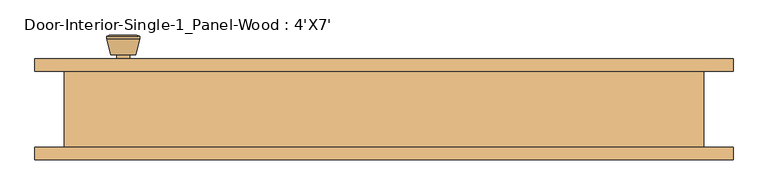
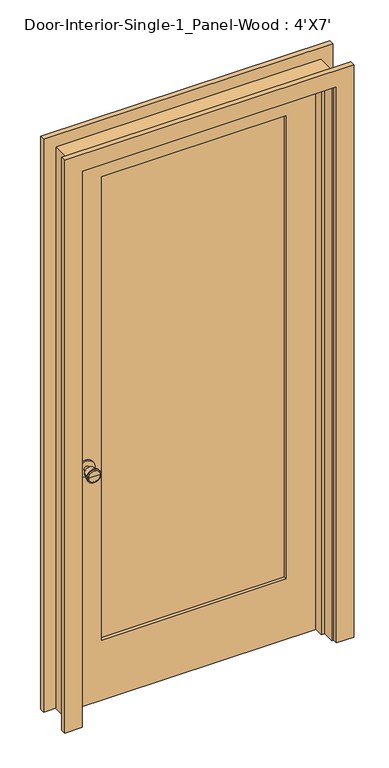
"""IFC4 building model written with IfcOpenShell, lengths in millimetres: door geometry, Door-Interior-Single-1_Panel-Wood : 4'X7'."""

from ifc_helpers import new_model, si_unit, point, frame, frame_2d, origin, place, context, project, spatial, polyline, circle_curve, trimmed, segment, composite_curve, outline, extrude, faceted_brep, source, transform, mapped, element, save
from ifc_brep_helpers import plane_surface, cylinder_surface, revolved_surface, advanced_brep


def door_interior_single_1_panel_wood_4_x7_3c6ab76a(model_context):
    return source(origin(), model_context, "Body", "SolidModel", [
        advanced_brep(
        [(-393.7, 13.05, 914.4), (-383.7, 13.05, 914.4), (-403.7, 13.05, 914.4), (-373.2241324, -35.95, 914.4), (-393.7, -35.95, 914.4), (-414.1758676, -35.95, 914.4), (-368.7, -34.1221319, 914.4), (-418.7, -34.1221319, 914.4), (-368.7, -30.6584537, 914.4), (-418.7, -30.6584537, 914.4), (-375.063764, -5.95, 914.4), (-412.336236, -5.95, 914.4), (-383.7, -5.95, 914.4), (-403.7, -5.95, 914.4)],
        [
            (0, 1),
            (1, 2, circle_curve(frame((-393.7, 13.05, 914.4), z_axis=(0.0, 1.0, 0.0), x_axis=(-1.0, 0.0, 0.0)), 10.0)),
            (2, 0),
            (2, 1, circle_curve(frame((-393.7, 13.05, 914.4), z_axis=(0.0, 1.0, 0.0), x_axis=(-1.0, 0.0, 0.0)), 10.0)),
            (3, 4),
            (4, 5),
            (5, 3, circle_curve(frame((-393.7, -35.95, 914.4), z_axis=(0.0, -1.0, 0.0), x_axis=(-1.0, 0.0, 0.0)), 20.4758676)),
            (3, 5, circle_curve(frame((-393.7, -35.95, 914.4), z_axis=(0.0, -1.0, 0.0), x_axis=(-1.0, 0.0, 0.0)), 20.4758676)),
            (6, 3),
            (5, 7),
            (7, 6, circle_curve(frame((-393.7, -34.1221319, 914.4), z_axis=(0.0, -1.0, 0.0), x_axis=(-1.0, 0.0, 0.0)), 25.0)),
            (6, 7, circle_curve(frame((-393.7, -34.1221319, 914.4), z_axis=(0.0, -1.0, 0.0), x_axis=(-1.0, 0.0, 0.0)), 25.0)),
            (8, 6),
            (7, 9),
            (9, 8, circle_curve(frame((-393.7, -30.6584537, 914.4), z_axis=(0.0, -1.0, 0.0), x_axis=(-1.0, 0.0, 0.0)), 25.0)),
            (8, 9, circle_curve(frame((-393.7, -30.6584537, 914.4), z_axis=(0.0, -1.0, 0.0), x_axis=(-1.0, 0.0, 0.0)), 25.0)),
            (10, 8),
            (9, 11),
            (11, 10, circle_curve(frame((-393.7, -5.95, 914.4), z_axis=(0.0, -1.0, 0.0), x_axis=(-1.0, 0.0, 0.0)), 18.636236)),
            (10, 11, circle_curve(frame((-393.7, -5.95, 914.4), z_axis=(0.0, -1.0, 0.0), x_axis=(-1.0, 0.0, 0.0)), 18.636236)),
            (12, 10),
            (11, 13),
            (13, 12, circle_curve(frame((-393.7, -5.95, 914.4), z_axis=(0.0, -1.0, 0.0), x_axis=(-1.0, 0.0, 0.0)), 10.0)),
            (12, 13, circle_curve(frame((-393.7, -5.95, 914.4), z_axis=(0.0, -1.0, 0.0), x_axis=(-1.0, 0.0, 0.0)), 10.0)),
            (1, 12),
            (13, 2),
        ],
        [
            plane_surface(frame((-393.7, 13.05, 914.4), z_axis=(0.0, 1.0, 0.0), x_axis=(-1.0, 0.0, 0.0))),
            plane_surface(frame((-393.7, -35.95, 914.4), z_axis=(0.0, -1.0, 0.0), x_axis=(-1.0, 0.0, 0.0))),
            revolved_surface(polyline([(-414.1758676, -35.95, 914.4), (-418.7, -34.1221319, 914.4)]), (-393.7, 13.05, 914.4), (0.0, 1.0, 0.0)),
            cylinder_surface(frame((-393.7, 13.05, 914.4), z_axis=(0.0, 1.0, 0.0), x_axis=(-1.0, 0.0, 0.0)), 25.0),
            revolved_surface(polyline([(-418.7, -30.6584537, 914.4), (-412.336236, -5.95, 914.4)]), (-393.7, 13.05, 914.4), (0.0, 1.0, 0.0)),
            plane_surface(frame((-393.7, -5.95, 914.4), z_axis=(0.0, 1.0, 0.0), x_axis=(-1.0, 0.0, 0.0))),
            cylinder_surface(frame((-393.7, 13.05, 914.4), z_axis=(0.0, 1.0, 0.0), x_axis=(-1.0, 0.0, 0.0)), 10.0),
        ],
        [
            (0, [[1, 2, 3]]),
            (0, [[-3, 4, -1]]),
            (1, [[5, 6, 7]]),
            (1, [[-6, -5, 8]]),
            (2, [[9, -7, 10, 11]]),
            (2, [[-10, -8, -9, 12]]),
            (3, [[13, -11, 14, 15]]),
            (3, [[-14, -12, -13, 16]]),
            (4, [[17, -15, 18, 19]]),
            (4, [[-18, -16, -17, 20]]),
            (5, [[21, -19, 22, 23]]),
            (5, [[-22, -20, -21, 24]]),
            (6, [[25, -23, 26, -2]]),
            (6, [[-26, -24, -25, -4]]),
        ],
    ),
        extrude(outline(composite_curve([segment(trimmed(circle_curve(frame_2d((914.4, -393.7)), 30.0), [point((914.4, -423.7))], [point((914.4, -363.7))], False, "CARTESIAN"), True, "CONTINUOUS"), segment(trimmed(circle_curve(frame_2d((914.4, -393.7)), 30.0), [point((914.4, -363.7))], [point((914.4, -423.7))], False, "CARTESIAN"), True, "CONTINUOUS")], self_intersect=False)), frame((0.0, 13.05, 0.0), z_axis=(0.0, 1.0, 0.0), x_axis=(0.0, 0.0, 1.0)), (0.0, 0.0, 1.0), 6.0),
        advanced_brep(
        [(-393.7, 59.975, 914.4), (-403.7, 59.975, 914.4), (-383.7, 59.975, 914.4), (-373.2241324, 108.975, 914.4), (-414.1758676, 108.975, 914.4), (-393.7, 108.975, 914.4), (-368.7, 107.1471319, 914.4), (-418.7, 107.1471319, 914.4), (-368.7, 103.6834537, 914.4), (-418.7, 103.6834537, 914.4), (-375.063764, 78.975, 914.4), (-412.336236, 78.975, 914.4), (-383.7, 78.975, 914.4), (-403.7, 78.975, 914.4)],
        [
            (0, 1),
            (1, 2, circle_curve(frame((-393.7, 59.975, 914.4), z_axis=(0.0, -1.0, 0.0), x_axis=(-1.0, 0.0, 0.0)), 10.0)),
            (2, 0),
            (2, 1, circle_curve(frame((-393.7, 59.975, 914.4), z_axis=(0.0, -1.0, 0.0), x_axis=(-1.0, 0.0, 0.0)), 10.0)),
            (3, 4, circle_curve(frame((-393.7, 108.975, 914.4), z_axis=(0.0, 1.0, 0.0), x_axis=(-1.0, 0.0, 0.0)), 20.4758676)),
            (4, 5),
            (5, 3),
            (4, 3, circle_curve(frame((-393.7, 108.975, 914.4), z_axis=(0.0, 1.0, 0.0), x_axis=(-1.0, 0.0, 0.0)), 20.4758676)),
            (6, 7, circle_curve(frame((-393.7, 107.1471319, 914.4), z_axis=(0.0, 1.0, 0.0), x_axis=(-1.0, 0.0, 0.0)), 25.0)),
            (7, 4),
            (3, 6),
            (7, 6, circle_curve(frame((-393.7, 107.1471319, 914.4), z_axis=(0.0, 1.0, 0.0), x_axis=(-1.0, 0.0, 0.0)), 25.0)),
            (8, 9, circle_curve(frame((-393.7, 103.6834537, 914.4), z_axis=(0.0, 1.0, 0.0), x_axis=(-1.0, 0.0, 0.0)), 25.0)),
            (9, 7),
            (6, 8),
            (9, 8, circle_curve(frame((-393.7, 103.6834537, 914.4), z_axis=(0.0, 1.0, 0.0), x_axis=(-1.0, 0.0, 0.0)), 25.0)),
            (10, 11, circle_curve(frame((-393.7, 78.975, 914.4), z_axis=(0.0, 1.0, 0.0), x_axis=(-1.0, 0.0, 0.0)), 18.636236)),
            (11, 9),
            (8, 10),
            (11, 10, circle_curve(frame((-393.7, 78.975, 914.4), z_axis=(0.0, 1.0, 0.0), x_axis=(-1.0, 0.0, 0.0)), 18.636236)),
            (12, 13, circle_curve(frame((-393.7, 78.975, 914.4), z_axis=(0.0, 1.0, 0.0), x_axis=(-1.0, 0.0, 0.0)), 10.0)),
            (13, 11),
            (10, 12),
            (13, 12, circle_curve(frame((-393.7, 78.975, 914.4), z_axis=(0.0, 1.0, 0.0), x_axis=(-1.0, 0.0, 0.0)), 10.0)),
            (1, 13),
            (12, 2),
        ],
        [
            plane_surface(frame((-393.7, 59.975, 914.4), z_axis=(0.0, -1.0, 0.0), x_axis=(-1.0, 0.0, 0.0))),
            plane_surface(frame((-393.7, 108.975, 914.4), z_axis=(0.0, 1.0, 0.0), x_axis=(-1.0, 0.0, 0.0))),
            revolved_surface(polyline([(-414.1758676, 108.975, 914.4), (-418.7, 107.1471319, 914.4)]), (-393.7, 59.975, 914.4), (0.0, -1.0, 0.0)),
            cylinder_surface(frame((-393.7, 59.975, 914.4), z_axis=(0.0, -1.0, 0.0), x_axis=(-1.0, 0.0, 0.0)), 25.0),
            revolved_surface(polyline([(-418.7, 103.6834537, 914.4), (-412.336236, 78.975, 914.4)]), (-393.7, 59.975, 914.4), (0.0, -1.0, 0.0)),
            plane_surface(frame((-393.7, 78.975, 914.4), z_axis=(0.0, -1.0, 0.0), x_axis=(-1.0, 0.0, 0.0))),
            cylinder_surface(frame((-393.7, 59.975, 914.4), z_axis=(0.0, -1.0, 0.0), x_axis=(-1.0, 0.0, 0.0)), 10.0),
        ],
        [
            (0, [[1, 2, 3]]),
            (0, [[-3, 4, -1]]),
            (1, [[5, 6, 7]]),
            (1, [[8, -7, -6]]),
            (2, [[9, 10, -5, 11]]),
            (2, [[12, -11, -8, -10]]),
            (3, [[13, 14, -9, 15]]),
            (3, [[16, -15, -12, -14]]),
            (4, [[17, 18, -13, 19]]),
            (4, [[20, -19, -16, -18]]),
            (5, [[21, 22, -17, 23]]),
            (5, [[24, -23, -20, -22]]),
            (6, [[-2, 25, -21, 26]]),
            (6, [[-4, -26, -24, -25]]),
        ],
    ),
        extrude(outline(composite_curve([segment(trimmed(circle_curve(frame_2d((914.4, -393.7)), 30.0), [point((914.4, -423.7))], [point((914.4, -363.7))], False, "CARTESIAN"), True, "CONTINUOUS"), segment(trimmed(circle_curve(frame_2d((914.4, -393.7)), 30.0), [point((914.4, -363.7))], [point((914.4, -423.7))], False, "CARTESIAN"), True, "CONTINUOUS")], self_intersect=False)), frame((0.0, 53.975, 0.0), z_axis=(0.0, 1.0, 0.0), x_axis=(0.0, 0.0, 1.0)), (0.0, 0.0, 1.0), 6.0),
        faceted_brep([(482.6, 53.975, 0.0), (482.6, -60.325, 0.0), (457.2, -60.325, 0.0), (457.2, -15.875, 0.0), (444.5, -15.875, 0.0), (444.5, 19.05, 0.0), (457.2, 19.05, 0.0), (457.2, 53.975, 0.0), (482.6, 53.975, 2159.0), (482.6, -60.325, 2159.0), (-482.6, -60.325, 2159.0), (-482.6, -60.325, 0.0), (-457.2, -60.325, 0.0), (-457.2, -60.325, 2133.6), (457.2, -60.325, 2133.6), (457.2, -15.875, 2133.6), (-457.2, -15.875, 2133.6), (-457.2, -15.875, 0.0), (-444.5, -15.875, 0.0), (-444.5, -15.875, 2120.9), (444.5, -15.875, 2120.9), (444.5, 19.05, 2120.9), (-444.5, 19.05, 2120.9), (-444.5, 19.05, 0.0), (-457.2, 19.05, 0.0), (-457.2, 19.05, 2133.6), (457.2, 19.05, 2133.6), (457.2, 53.975, 2133.6), (-457.2, 53.975, 2133.6), (-457.2, 53.975, 0.0), (-482.6, 53.975, 0.0), (-482.6, 53.975, 2159.0)], [[[0, 1, 2, 3, 4, 5, 6, 7]], [[1, 0, 8, 9]], [[2, 1, 9, 10, 11, 12, 13, 14]], [[3, 2, 14, 15]], [[4, 3, 15, 16, 17, 18, 19, 20]], [[5, 4, 20, 21]], [[6, 5, 21, 22, 23, 24, 25, 26]], [[7, 6, 26, 27]], [[0, 7, 27, 28, 29, 30, 31, 8]], [[9, 8, 31, 10]], [[15, 14, 13, 16]], [[21, 20, 19, 22]], [[27, 26, 25, 28]], [[30, 29, 24, 23, 18, 17, 12, 11]], [[10, 31, 30, 11]], [[16, 13, 12, 17]], [[22, 19, 18, 23]], [[28, 25, 24, 29]]]),
        extrude(outline(polyline([(2133.6, -457.2), (0.0, -457.2), (0.0, 457.2), (2133.6, 457.2), (2133.6, -457.2)]), holes=[polyline([(2014.5375, -336.55), (2014.5375, 336.55), (231.775, 336.55), (231.775, -336.55), (2014.5375, -336.55)])]), frame((0.0, 19.05, 0.0), z_axis=(0.0, 1.0, 0.0), x_axis=(0.0, 0.0, 1.0)), (0.0, 0.0, 1.0), 34.925),
        extrude(outline(polyline([(336.55, 30.6916667), (-336.55, 30.6916667), (-336.55, 42.3333333), (336.55, 42.3333333), (336.55, 30.6916667)])), frame((0.0, 0.0, 231.775), z_axis=(0.0, 0.0, 1.0), x_axis=(1.0, 0.0, 0.0)), (0.0, 0.0, 1.0), 1782.7625),
        extrude(outline(polyline([(0.0, 463.55), (0.0, 527.05), (2203.45, 527.05), (2203.45, -527.05), (0.0, -527.05), (0.0, -463.55), (2139.95, -463.55), (2139.95, 463.55), (0.0, 463.55)])), frame((0.0, 53.975, 0.0), z_axis=(0.0, 1.0, 0.0), x_axis=(0.0, 0.0, 1.0)), (0.0, 0.0, 1.0), 19.05),
        extrude(outline(polyline([(0.0, 463.55), (0.0, 527.05), (2203.45, 527.05), (2203.45, -527.05), (0.0, -527.05), (0.0, -463.55), (2139.95, -463.55), (2139.95, 463.55), (0.0, 463.55)])), frame((0.0, -79.375, 0.0), z_axis=(0.0, 1.0, 0.0), x_axis=(0.0, 0.0, 1.0)), (0.0, 0.0, 1.0), 19.05),
    ])


if __name__ == "__main__":
    model = new_model("IFC4")
    model_context = context("Model", 3, world=origin())
    ifc_project = project(units=[si_unit("LENGTHUNIT", "METRE", prefix="MILLI")], contexts=[model_context])
    site = spatial("IfcSite", under=ifc_project)
    building = spatial("IfcBuilding", under=site)
    placement = place(None, origin())
    door_interior_single_1_panel_wood_4_x7_shape = door_interior_single_1_panel_wood_4_x7_3c6ab76a(model_context)
    element("IfcDoor", 1, ObjectType="Door-Interior-Single-1_Panel-Wood : 4'X7'", at=placement, inside=building, context=model_context, shape_type="MappedRepresentation", body=[
        mapped(door_interior_single_1_panel_wood_4_x7_shape, transform((0.0, 0.0, 0.0), x_axis=(1.0, 0.0, 0.0), y_axis=(0.0, 1.0, 0.0), z_axis=(0.0, 0.0, 1.0))),
    ])
    save(model, "model.ifc")

# Revit data of these elements
# Type "Door-Interior-Single-1_Panel-Wood : 4'X7'"
#   Type Mark = "9"
#   Assembly Code = "C1020300"
#   Analytic Construction = "Wooden"
#   Top Rail = 0' - 4 11/16"
#   Thickness = 0' - 1 3/8"
#   Thermal Resistance (R) = 2.5876 (h·ft²·°F)/BTU
#   Swing Angle [instance default] = 90.00°
#   Stiles = 0' - 4 3/4"
#   Rough Width = 3' - 2"
#   Rough Height = 7' - 1"
#   Height = 7' - 0"
#   Width = 3' - 0"
#   Heat Transfer Coefficient (U) = 0.3865 BTU/(h·ft²·°F)
#   Bottom Rail = 0' - 9 1/8"
#   Trim Material = Cherry
#   Panel Material = Cherry
#   Frame Material = Cherry
#   Door Handle Material = Aluminum
#   Visual Light Transmittance = 0
#   Solar Heat Gain Coefficient = 0
#   Wall Closure = (empty or 0)
#   Function = (empty or 0)
# Element 1 (IfcDoor, "Door-Interior-Single-1_Panel-Wood : 4'X7'")
#   Materials on its faces: "Cherry", "Aluminum"
# Materials
#   "Cherry": class "Wood", colour RGB 226 177 128, transparency 0, Description = "Prunus Serotina", Cost = 0
#   "Aluminum": class "Metal", colour RGB 247 247 247, transparency 0, Description = "Aluminum 6061", Cost = 0
